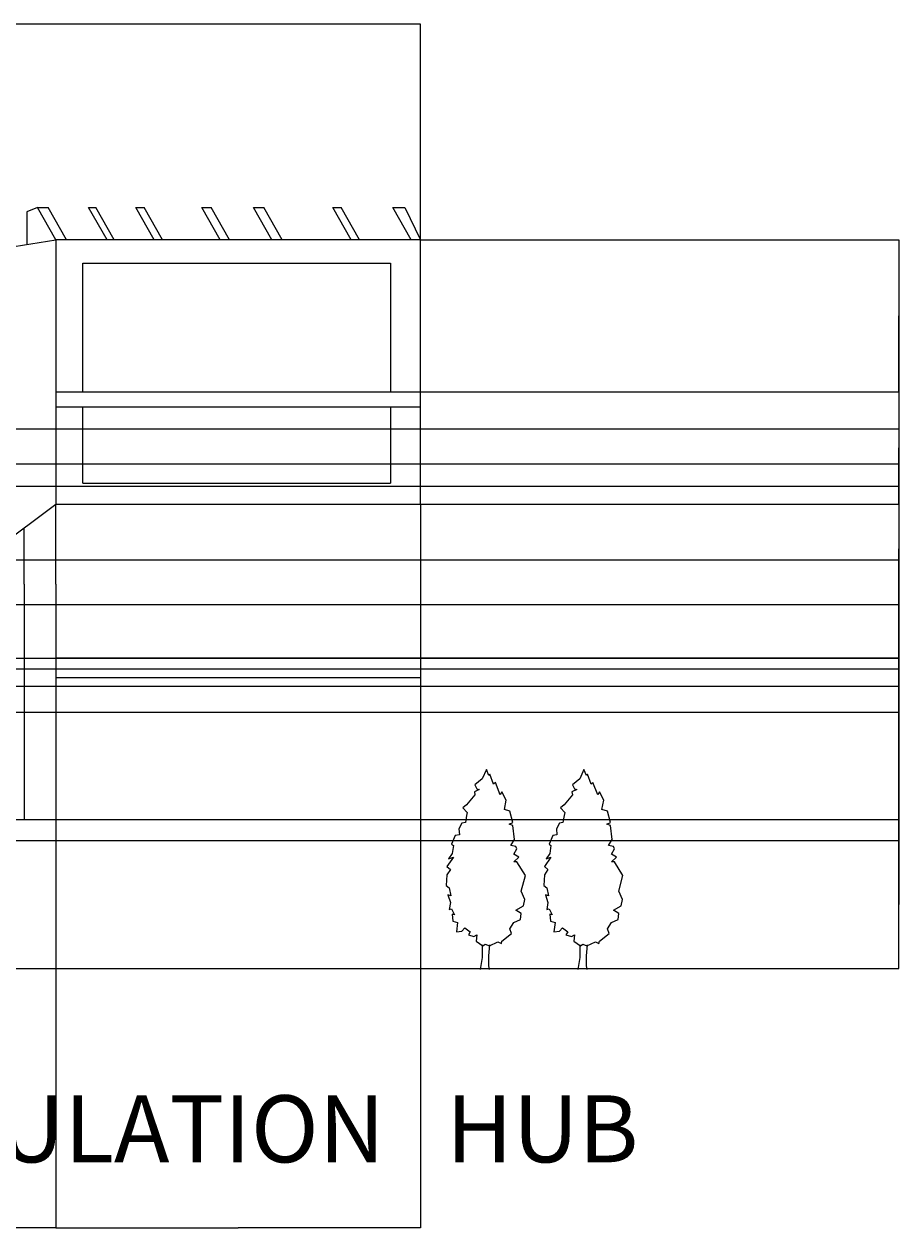
# Model space of a CAD drawing. Units: inches. Extents: x -32109 to 33221, y -19197 to 7608.
# Tile 24 of 25: x 26633 to 33221, y -13530 to -4467. Entities that reach past the tile are written whole.
import ezdxf

# ---------------------------------------------------------------- set-up
doc = ezdxf.new("R2010")
doc.units = ezdxf.units.IN
doc.header["$MEASUREMENT"] = 0
for name, color, linetype, lineweight in [('A-ANNO-DIMS', 2, 'Continuous', 18), ('A-ANNO-TEXT', 7, 'Continuous', 25), ('A-ELEV', 7, 'Continuous', 25), ('L-PLNT', 3, 'Continuous', 13)]:
    doc.layers.add(name, color=color, linetype=linetype, lineweight=lineweight)
doc.styles.get("Standard").update_dxf_attribs({"font": 'arial.ttf'})
doc.dimstyles.get("Standard").update_dxf_attribs({"dimtxt": 0.18, "dimasz": 0.18, "dimexe": 0.18, "dimexo": 0.0625, "dimgap": 0.09, "dimtad": 0, "dimtih": 1, "dimtoh": 1, "dimdec": 4, "dimzin": 0, "dimdsep": 46, "dimtxsty": 'Standard', "dimcen": 0.09, "dimadec": 0, "dimazin": 0, "dimtfac": 1, "dimtdec": 4, "dimtofl": 0, "dimtmove": 0, "dimatfit": 3, "dimfxl": 1, "dimtolj": 1, "dimtzin": 0, "dimarcsym": 0})

# ---------------------------------------------------------------- blocks, each defined once
blk = doc.blocks.new('*U2')
blk.add_lwpolyline([(-2.75400000000036, 191.699), (-6.7800000000002, 182.8509999999996), (-13.68200000000024, 176.9529999999995), (-11.95600000000013, 173.2659999999996), (-9.655999999999949, 172.529), (-14.25700000000006, 170.317), (-13.68200000000024, 167.3679999999999), (-21.73300000000017, 157.7829999999999), (-25.1840000000002, 154.8340000000003), (-21.15800000000036, 150.4099999999998), (-21.73300000000017, 147.4609999999998), (-22.88400000000001, 140.8249999999998), (-26.33400000000029, 140.087), (-29.21000000000004, 134.9259999999995), (-28.63499999999977, 129.0279999999998), (-32.66100000000006, 128.2909999999997), (-36.11099999999988, 120.1799999999998), (-34.38599999999997, 118.7059999999997), (-35.53600000000006, 111.3329999999996), (-38.98700000000008, 106.1709999999998), (-34.38599999999997, 107.6459999999997), (-40.71199999999999, 98.79799999999977), (-37.26099999999997, 95.8489999999997), (-40.71199999999999, 90.68799999999965), (-41.28700000000026, 80.36599999999999), (-38.41200000000026, 78.154), (-36.68600000000015, 70.78099999999995), (-39.5619999999999, 71.51799999999957), (-37.26099999999997, 64.14499999999998), (-38.41200000000026, 57.50899999999956), (-36.11099999999988, 58.24699999999984), (-33.23599999999988, 52.3479999999995), (-35.53600000000006, 53.08599999999978), (-34.96100000000024, 46.44999999999981), (-30.36000000000013, 44.9749999999999), (-31.50999999999977, 36.1279999999997), (-26.33400000000029, 36.86499999999978), (-23.45900000000029, 39.81399999999985), (-18.28300000000036, 36.1279999999997), (-20.00800000000027, 33.17799999999988), (-14.83199999999988, 31.70399999999972), (-11.95600000000013, 33.17799999999988), (-12.53099999999995, 27.27999999999975), (-6.204999999999927, 22.85599999999977), (-3.9050000000002, 24.33099999999968), (0.1209999999996398, 22.85599999999977), (8.172999999999774, 26.54299999999967), (11.62399999999979, 25.06799999999976), (12.19900000000007, 27.27999999999975), (21.40000000000009, 34.6529999999998), (19.67500000000018, 39.07699999999977), (23.70099999999957, 44.9749999999999), (30.02700000000004, 47.92399999999997), (30.60199999999986, 53.82299999999986), (25.42599999999993, 56.77199999999993), (32.90299999999979, 61.19599999999991), (34.05299999999988, 67.0939999999996), (30.60199999999986, 75.20499999999993), (34.6279999999997, 89.95100000000002), (26.57599999999957, 103.2219999999997), (23.70099999999957, 103.2219999999997), (28.30199999999968, 107.6459999999997), (23.70099999999957, 110.5949999999998), (26.57599999999957, 115.7559999999994), (25.42599999999993, 117.9679999999998), (20.82499999999982, 118.7059999999997), (24.27599999999984, 124.6040000000002), (22.55099999999993, 137.8759999999997), (19.09999999999991, 139.3499999999999), (22.55099999999993, 140.8249999999998), (19.67500000000018, 151.884), (14.49899999999979, 153.3589999999999), (16.22400000000016, 162.2069999999999), (12.19900000000007, 170.317), (10.47299999999995, 167.3679999999999), (5.871999999999843, 179.1649999999999), (4.146999999999934, 177.69), (0.6959999999999127, 187.2749999999996), (-0.4540000000001783, 185.7999999999997)], close=True)
for points in [[(-6.813000000000101, 23.66899999999987), (-6.813000000000101, 11.66899999999987), (-8.626999999999953, 0)], [(0.3869999999997162, 23.66899999999987), (-0.5760000000000219, 13.27099999999973), (-0.5760000000000219, 3.685999999999694), (0, 0)]]:
    blk.add_lwpolyline(points)
blk = doc.blocks.new('*D16')
at = {"layer": 'A-ANNO-DIMS', "color": 0, "lineweight": -2, "transparency": 16777216}
for p, q in [((7931.85712, -8929.002357), (7931.85712, -4467.086268999999)), ((7932.03712, -4467.266268999999), (18774.66361096794, -4467.266268999999)), ((29618.150443, -4467.266268999999), (18775.52395203206, -4467.266268999999)), ((29618.330443, -6090.731526999999), (29618.330443, -4467.086268999999))]:
    blk.add_line(p, q, dxfattribs=at)
at = {"layer": 'A-ANNO-DIMS', "color": 0, "transparency": 16777216}
for points in [[(7932.03712, -4467.236268999999), (7932.03712, -4467.296269), (7931.85712, -4467.266268999999)], [(29618.150443, -4467.236268999999), (29618.150443, -4467.296269), (29618.330443, -4467.266268999999)]]:
    blk.add_solid(points, dxfattribs=at)
at = {"layer": 'Defpoints', "color": 0, "transparency": 16777216}
for p in [(29618.330443, -4467.266268999999), (29618.330443, -6090.794027), (7931.85712, -8929.064857)]:
    blk.add_point(p, dxfattribs=at)
at = {"layer": 'A-ANNO-DIMS', "color": 0, "transparency": 16777216, "insert": (18775.0937815, -4467.266268999999), "char_height": 0.18, "attachment_point": 5}
blk.add_mtext('\\A1;21686', dxfattribs=at)
blk = doc.blocks.new('*D17')
at = {"layer": 'A-ANNO-DIMS', "color": 0, "lineweight": -2, "transparency": 16777216}
for p, q in [((29618.39294300002, -6090.794027000002), (33221.11530000003, -6090.794027000001)), ((33220.93530000003, -6090.974027000001), (33220.93530000003, -8833.116883862214)), ((33220.93530000003, -11575.623547), (33220.93530000003, -8833.48069013779)), ((8978.174905000003, -11575.803547), (33221.11530000003, -11575.803547))]:
    blk.add_line(p, q, dxfattribs=at)
at = {"layer": 'A-ANNO-DIMS', "color": 0, "transparency": 16777216}
for points in [[(33220.90530000003, -6090.974027000001), (33220.96530000003, -6090.974027000001), (33220.93530000003, -6090.794027000001)], [(33220.90530000003, -11575.623547), (33220.96530000003, -11575.623547), (33220.93530000003, -11575.803547)]]:
    blk.add_solid(points, dxfattribs=at)
at = {"layer": 'Defpoints', "color": 0, "transparency": 16777216}
for p in [(29618.33044300001, -6090.794027000002), (8978.112405000002, -11575.803547), (33220.93530000003, -11575.803547)]:
    blk.add_point(p, dxfattribs=at)
at = {"layer": 'A-ANNO-DIMS', "color": 0, "transparency": 16777216, "insert": (33220.93530000002, -8833.298787000009), "char_height": 0.18, "attachment_point": 5}
blk.add_mtext('\\A1;5485', dxfattribs=at)
blk = doc.blocks.new('*D140')
at = {"layer": 'A-ANNO-DIMS', "color": 0, "lineweight": -2, "transparency": 16777216}
for p, q in [((24779.369992, -11575.866047), (24779.369992, -13529.670166)), ((26872.591633, -11575.866047), (26872.591633, -13529.670166)), ((24779.549992, -13529.490166), (25825.51656966234, -13529.490166)), ((26872.411633, -13529.490166), (25826.44505533765, -13529.490166))]:
    blk.add_line(p, q, dxfattribs=at)
at = {"layer": 'A-ANNO-DIMS', "color": 0, "transparency": 16777216}
for points in [[(24779.549992, -13529.460166), (24779.549992, -13529.520166), (24779.369992, -13529.490166)], [(26872.411633, -13529.460166), (26872.411633, -13529.520166), (26872.591633, -13529.490166)]]:
    blk.add_solid(points, dxfattribs=at)
at = {"layer": 'Defpoints', "color": 0, "transparency": 16777216}
for p in [(24779.369992, -11575.803547), (26872.591633, -11575.803547), (26872.591633, -13529.490166)]:
    blk.add_point(p, dxfattribs=at)
at = {"layer": 'A-ANNO-DIMS', "color": 0, "transparency": 16777216, "insert": (25825.9808125, -13529.490166), "char_height": 0.18, "attachment_point": 5}
blk.add_mtext('\\A1;2093.2', dxfattribs=at)
blk = doc.blocks.new('*D141')
at = {"layer": 'A-ANNO-DIMS', "color": 0, "lineweight": -2, "transparency": 16777216}
for p, q in [((26872.591633, -11575.866047), (26872.591633, -13529.670166)), ((29618.330443, -11575.866047), (29618.330443, -13529.670166)), ((26872.771633, -13529.490166), (28245.10079243383, -13529.490166)), ((29618.150443, -13529.490166), (28245.82128356617, -13529.490166))]:
    blk.add_line(p, q, dxfattribs=at)
at = {"layer": 'A-ANNO-DIMS', "color": 0, "transparency": 16777216}
for points in [[(26872.771633, -13529.460166), (26872.771633, -13529.520166), (26872.591633, -13529.490166)], [(29618.150443, -13529.460166), (29618.150443, -13529.520166), (29618.330443, -13529.490166)]]:
    blk.add_solid(points, dxfattribs=at)
at = {"layer": 'Defpoints', "color": 0, "transparency": 16777216}
for p in [(26872.591633, -11575.803547), (29618.330443, -11575.803547), (29618.330443, -13529.490166)]:
    blk.add_point(p, dxfattribs=at)
at = {"layer": 'A-ANNO-DIMS', "color": 0, "transparency": 16777216, "insert": (28245.461038, -13529.490166), "char_height": 0.18, "attachment_point": 5}
blk.add_mtext('\\A1;2746', dxfattribs=at)
blk = doc.blocks.new('*D142')
at = {"layer": 'A-ANNO-DIMS', "color": 0, "lineweight": -2, "transparency": 16777216}
for p, q in [((19422.79326, -7777.039673000004), (33221.11530000003, -7777.039673000001)), ((33220.93530000003, -7777.219673000002), (33220.93530000003, -9676.23964547067)), ((33220.93530000003, -11575.623547), (33220.93530000003, -9676.603574529332)), ((19422.79326, -11575.803547), (33221.11530000003, -11575.803547))]:
    blk.add_line(p, q, dxfattribs=at)
at = {"layer": 'A-ANNO-DIMS', "color": 0, "transparency": 16777216}
for points in [[(33220.90530000003, -7777.219673000002), (33220.96530000003, -7777.219673000002), (33220.93530000003, -7777.039673000001)], [(33220.90530000003, -11575.623547), (33220.96530000003, -11575.623547), (33220.93530000003, -11575.803547)]]:
    blk.add_solid(points, dxfattribs=at)
at = {"layer": 'Defpoints', "color": 0, "transparency": 16777216}
for p in [(19422.73076, -7777.039673000004), (19422.73076, -11575.803547), (33220.93530000003, -11575.803547)]:
    blk.add_point(p, dxfattribs=at)
at = {"layer": 'A-ANNO-DIMS', "color": 0, "transparency": 16777216, "insert": (33220.93530000002, -9676.421610000009), "char_height": 0.18, "attachment_point": 5}
blk.add_mtext('\\A1;3799', dxfattribs=at)
blk = doc.blocks.new('*D143')
at = {"layer": 'A-ANNO-DIMS', "color": 0, "lineweight": -2, "transparency": 16777216}
for p, q in [((23344.28486700001, -9241.758819000004), (33221.11530000003, -9241.758819000002)), ((33220.93530000003, -9241.938819000003), (33220.93530000003, -10408.59921847067)), ((33220.93530000003, -11575.623547), (33220.93530000003, -10408.96314752933)), ((23344.28486700001, -11575.803547), (33221.11530000003, -11575.803547))]:
    blk.add_line(p, q, dxfattribs=at)
at = {"layer": 'A-ANNO-DIMS', "color": 0, "transparency": 16777216}
for points in [[(33220.90530000003, -9241.938819000003), (33220.96530000003, -9241.938819000003), (33220.93530000003, -9241.758819000002)], [(33220.90530000003, -11575.623547), (33220.96530000003, -11575.623547), (33220.93530000003, -11575.803547)]]:
    blk.add_solid(points, dxfattribs=at)
at = {"layer": 'Defpoints', "color": 0, "transparency": 16777216}
for p in [(23344.222367, -9241.758819000004), (23344.222367, -11575.803547), (33220.93530000003, -11575.803547)]:
    blk.add_point(p, dxfattribs=at)
at = {"layer": 'A-ANNO-DIMS', "color": 0, "transparency": 16777216, "insert": (33220.93530000002, -10408.78118300001), "char_height": 0.18, "attachment_point": 5}
blk.add_mtext('\\A1;2334', dxfattribs=at)
blk = doc.blocks.new('*D144')
at = {"layer": 'A-ANNO-DIMS', "color": 0, "lineweight": -2, "transparency": 16777216}
for p, q in [((22344.03431300001, -7946.222949000004), (33221.11530000003, -7946.222949000001)), ((33220.93530000003, -7946.402949000002), (33220.93530000003, -8593.808980862214)), ((33220.93530000003, -9241.578819000002), (33220.93530000003, -8594.172787137792)), ((22344.03431300001, -9241.758819000004), (33221.11530000003, -9241.758819000002))]:
    blk.add_line(p, q, dxfattribs=at)
at = {"layer": 'A-ANNO-DIMS', "color": 0, "transparency": 16777216}
for points in [[(33220.90530000003, -7946.402949000002), (33220.96530000003, -7946.402949000002), (33220.93530000003, -7946.222949000001)], [(33220.90530000003, -9241.578819000002), (33220.96530000003, -9241.578819000002), (33220.93530000003, -9241.758819000002)]]:
    blk.add_solid(points, dxfattribs=at)
at = {"layer": 'Defpoints', "color": 0, "transparency": 16777216}
for p in [(22343.97181300001, -7946.222949000004), (22343.97181300001, -9241.758819000004), (33220.93530000003, -9241.758819000002)]:
    blk.add_point(p, dxfattribs=at)
at = {"layer": 'A-ANNO-DIMS', "color": 0, "transparency": 16777216, "insert": (33220.93530000002, -8593.99088400001), "char_height": 0.18, "attachment_point": 5}
blk.add_mtext('\\A1;1295.5', dxfattribs=at)
blk = doc.blocks.new('*D145')
at = {"layer": 'A-ANNO-DIMS', "color": 0, "lineweight": -2, "transparency": 16777216}
for p, q in [((20542.28536700001, -9450.896666000002), (33221.11530000003, -9450.896666000002)), ((33220.93530000003, -9451.076666000004), (33220.93530000003, -10513.16820336221)), ((33220.93530000003, -11575.623547), (33220.93530000003, -10513.53200963779)), ((20542.28536700001, -11575.803547), (33221.11530000003, -11575.803547))]:
    blk.add_line(p, q, dxfattribs=at)
at = {"layer": 'A-ANNO-DIMS', "color": 0, "transparency": 16777216}
for points in [[(33220.90530000003, -9451.076666000004), (33220.96530000003, -9451.076666000004), (33220.93530000003, -9450.896666000002)], [(33220.90530000003, -11575.623547), (33220.96530000003, -11575.623547), (33220.93530000003, -11575.803547)]]:
    blk.add_solid(points, dxfattribs=at)
at = {"layer": 'Defpoints', "color": 0, "transparency": 16777216}
for p in [(20542.22286700001, -9450.896666000002), (20542.22286700001, -11575.803547), (33220.93530000003, -11575.803547)]:
    blk.add_point(p, dxfattribs=at)
at = {"layer": 'A-ANNO-DIMS', "color": 0, "transparency": 16777216, "insert": (33220.93530000002, -10513.35010650001), "char_height": 0.18, "attachment_point": 5}
blk.add_mtext('\\A1;2125', dxfattribs=at)
blk = doc.blocks.new('*D147')
at = {"layer": 'A-ANNO-DIMS', "color": 0, "lineweight": -2, "transparency": 16777216}
for p, q in [((25729.07058000001, -7514.357851000004), (33221.11530000003, -7514.357851000003)), ((33220.93530000003, -7514.537851000003), (33220.93530000003, -8416.924501362213)), ((33220.93530000003, -9319.674958000001), (33220.93530000003, -8417.288307637791)), ((23373.8343, -9319.854958000004), (33221.11530000003, -9319.854958000002))]:
    blk.add_line(p, q, dxfattribs=at)
at = {"layer": 'A-ANNO-DIMS', "color": 0, "transparency": 16777216}
for points in [[(33220.90530000003, -7514.537851000003), (33220.96530000003, -7514.537851000003), (33220.93530000003, -7514.357851000003)], [(33220.90530000003, -9319.674958000001), (33220.96530000003, -9319.674958000001), (33220.93530000003, -9319.854958000002)]]:
    blk.add_solid(points, dxfattribs=at)
at = {"layer": 'Defpoints', "color": 0, "transparency": 16777216}
for p in [(25729.00808000002, -7514.357851000004), (33220.93530000003, -7514.357851000003), (23373.77180000001, -9319.854958000004)]:
    blk.add_point(p, dxfattribs=at)
at = {"layer": 'A-ANNO-DIMS', "color": 0, "transparency": 16777216, "insert": (33220.93530000002, -8417.10640450001), "char_height": 0.18, "attachment_point": 5}
blk.add_mtext('\\A1;1805.5', dxfattribs=at)
blk = doc.blocks.new('*D149')
at = {"layer": 'A-ANNO-DIMS', "color": 0, "lineweight": -2, "transparency": 16777216}
for p, q in [((24743.24553300002, -8499.326661000003), (33221.11530000003, -8499.326661000001)), ((33220.93530000003, -8499.506661000001), (33220.93530000003, -8667.240442470671)), ((33220.93530000003, -8835.338153000002), (33220.93530000003, -8667.604371529334)), ((24743.24553300002, -8835.518153000005), (33221.11530000003, -8835.518153000003))]:
    blk.add_line(p, q, dxfattribs=at)
at = {"layer": 'A-ANNO-DIMS', "color": 0, "transparency": 16777216}
for points in [[(33220.90530000003, -8499.506661000001), (33220.96530000003, -8499.506661000001), (33220.93530000003, -8499.326661000001)], [(33220.90530000003, -8835.338153000002), (33220.96530000003, -8835.338153000002), (33220.93530000003, -8835.518153000003)]]:
    blk.add_solid(points, dxfattribs=at)
at = {"layer": 'Defpoints', "color": 0, "transparency": 16777216}
for p in [(24743.18303300002, -8499.326661000003), (33220.93530000003, -8499.326661000001), (24743.18303300002, -8835.518153000005)]:
    blk.add_point(p, dxfattribs=at)
at = {"layer": 'A-ANNO-DIMS', "color": 0, "transparency": 16777216, "insert": (33220.93530000002, -8667.422407000007), "char_height": 0.18, "attachment_point": 5}
blk.add_mtext('\\A1;336.2', dxfattribs=at)
blk = doc.blocks.new('*D150')
at = {"layer": 'A-ANNO-DIMS', "color": 0, "lineweight": -2, "transparency": 16777216}
for p, q in [((24779.43249200002, -9646.283758000003), (33221.11530000003, -9646.283758000001)), ((33220.93530000003, -9646.463758000002), (33220.93530000003, -10050.72724947067)), ((33220.93530000003, -10455.35467), (33220.93530000003, -10051.09117852933)), ((24779.43249200002, -10455.53467), (33221.11530000003, -10455.53467))]:
    blk.add_line(p, q, dxfattribs=at)
at = {"layer": 'A-ANNO-DIMS', "color": 0, "transparency": 16777216}
for points in [[(33220.90530000003, -9646.463758000002), (33220.96530000003, -9646.463758000002), (33220.93530000003, -9646.283758000001)], [(33220.90530000003, -10455.35467), (33220.96530000003, -10455.35467), (33220.93530000003, -10455.53467)]]:
    blk.add_solid(points, dxfattribs=at)
at = {"layer": 'Defpoints', "color": 0, "transparency": 16777216}
for p in [(24779.36999200001, -9646.283758000003), (24779.36999200001, -10455.53467), (33220.93530000003, -10455.53467)]:
    blk.add_point(p, dxfattribs=at)
at = {"layer": 'A-ANNO-DIMS', "color": 0, "transparency": 16777216, "insert": (33220.93530000002, -10050.90921400001), "char_height": 0.18, "attachment_point": 5}
blk.add_mtext('\\A1;809.3', dxfattribs=at)
blk = doc.blocks.new('*D151')
at = {"layer": 'A-ANNO-DIMS', "color": 0, "lineweight": -2, "transparency": 16777216}
for p, q in [((24779.43249200002, -10455.53467), (33221.11530000003, -10455.53467)), ((33220.93530000003, -10455.71467), (33220.93530000003, -11015.48714397067)), ((33220.93530000003, -11575.623547), (33220.93530000003, -11015.85107302933)), ((24779.43249200002, -11575.803547), (33221.11530000003, -11575.803547))]:
    blk.add_line(p, q, dxfattribs=at)
at = {"layer": 'A-ANNO-DIMS', "color": 0, "transparency": 16777216}
for points in [[(33220.90530000003, -10455.71467), (33220.96530000003, -10455.71467), (33220.93530000003, -10455.53467)], [(33220.90530000003, -11575.623547), (33220.96530000003, -11575.623547), (33220.93530000003, -11575.803547)]]:
    blk.add_solid(points, dxfattribs=at)
at = {"layer": 'Defpoints', "color": 0, "transparency": 16777216}
for p in [(24779.36999200001, -10455.53467), (24779.36999200001, -11575.803547), (33220.93530000003, -11575.803547)]:
    blk.add_point(p, dxfattribs=at)
at = {"layer": 'A-ANNO-DIMS', "color": 0, "transparency": 16777216, "insert": (33220.93530000002, -11015.66910850001), "char_height": 0.18, "attachment_point": 5}
blk.add_mtext('\\A1;1120.3', dxfattribs=at)
blk = doc.blocks.new('*D153')
at = {"layer": 'A-ANNO-DIMS', "color": 0, "lineweight": -2, "transparency": 16777216}
for p, q in [((29618.39294300002, -10614.330461), (33221.11530000003, -10614.330461)), ((33220.93530000003, -10614.510461), (33220.93530000003, -11094.88510086221)), ((33220.93530000003, -11575.623547), (33220.93530000003, -11095.24890713779)), ((29618.39294300002, -11575.803547), (33221.11530000003, -11575.803547))]:
    blk.add_line(p, q, dxfattribs=at)
at = {"layer": 'A-ANNO-DIMS', "color": 0, "transparency": 16777216}
for points in [[(33220.90530000003, -10614.510461), (33220.96530000003, -10614.510461), (33220.93530000003, -10614.330461)], [(33220.90530000003, -11575.623547), (33220.96530000003, -11575.623547), (33220.93530000003, -11575.803547)]]:
    blk.add_solid(points, dxfattribs=at)
at = {"layer": 'Defpoints', "color": 0, "transparency": 16777216}
for p in [(29618.33044300001, -10614.330461), (33220.93530000003, -10614.330461), (29618.33044300001, -11575.803547)]:
    blk.add_point(p, dxfattribs=at)
at = {"layer": 'A-ANNO-DIMS', "color": 0, "transparency": 16777216, "insert": (33220.93530000002, -11095.06700400001), "char_height": 0.18, "attachment_point": 5}
blk.add_mtext('\\A1;961.5', dxfattribs=at)
blk = doc.blocks.new('*D154')
at = {"layer": 'A-ANNO-DIMS', "color": 0, "lineweight": -2, "transparency": 16777216}
for p, q in [((29618.39294300002, -9238.017771000004), (33221.11530000003, -9238.017771000004)), ((33220.93530000003, -9238.197771000005), (33220.93530000003, -9925.992151470673)), ((33220.93530000003, -10614.150461), (33220.93530000003, -9926.356080529336)), ((29618.39294300002, -10614.330461), (33221.11530000003, -10614.330461))]:
    blk.add_line(p, q, dxfattribs=at)
at = {"layer": 'A-ANNO-DIMS', "color": 0, "transparency": 16777216}
for points in [[(33220.90530000003, -9238.197771000005), (33220.96530000003, -9238.197771000005), (33220.93530000003, -9238.017771000004)], [(33220.90530000003, -10614.150461), (33220.96530000003, -10614.150461), (33220.93530000003, -10614.330461)]]:
    blk.add_solid(points, dxfattribs=at)
at = {"layer": 'Defpoints', "color": 0, "transparency": 16777216}
for p in [(29618.33044300001, -9238.017771000004), (33220.93530000003, -9238.017771000004), (29618.33044300001, -10614.330461)]:
    blk.add_point(p, dxfattribs=at)
at = {"layer": 'A-ANNO-DIMS', "color": 0, "transparency": 16777216, "insert": (33220.93530000002, -9926.174116000013), "char_height": 0.18, "attachment_point": 5}
blk.add_mtext('\\A1;1376.3', dxfattribs=at)
blk = doc.blocks.new('*D155')
at = {"layer": 'A-ANNO-DIMS', "color": 0, "lineweight": -2, "transparency": 16777216}
for p, q in [((29618.39294300002, -8080.142133000004), (33221.11530000003, -8080.142133000002)), ((33220.93530000003, -8080.322133000002), (33220.93530000003, -8658.898048862215)), ((33220.93530000003, -9237.837771000004), (33220.93530000003, -8659.261855137793)), ((29618.39294300002, -9238.017771000004), (33221.11530000003, -9238.017771000004))]:
    blk.add_line(p, q, dxfattribs=at)
at = {"layer": 'A-ANNO-DIMS', "color": 0, "transparency": 16777216}
for points in [[(33220.90530000003, -8080.322133000002), (33220.96530000003, -8080.322133000002), (33220.93530000003, -8080.142133000002)], [(33220.90530000003, -9237.837771000004), (33220.96530000003, -9237.837771000004), (33220.93530000003, -9238.017771000004)]]:
    blk.add_solid(points, dxfattribs=at)
at = {"layer": 'Defpoints', "color": 0, "transparency": 16777216}
for p in [(29618.33044300001, -8080.142133000004), (33220.93530000003, -8080.142133000002), (29618.33044300001, -9238.017771000004)]:
    blk.add_point(p, dxfattribs=at)
at = {"layer": 'A-ANNO-DIMS', "color": 0, "transparency": 16777216, "insert": (33220.93530000002, -8659.079952000011), "char_height": 0.18, "attachment_point": 5}
blk.add_mtext('\\A1;1157.9', dxfattribs=at)
blk = doc.blocks.new('*D156')
at = {"layer": 'A-ANNO-DIMS', "color": 0, "lineweight": -2, "transparency": 16777216}
for p, q in [((29618.39294300002, -7235.783167000004), (33221.11530000003, -7235.783167000002)), ((33220.93530000003, -7235.963167000003), (33220.93530000003, -7657.780746862214)), ((33220.93530000003, -8079.962133000002), (33220.93530000003, -7658.144553137794)), ((29618.39294300002, -8080.142133000004), (33221.11530000003, -8080.142133000002))]:
    blk.add_line(p, q, dxfattribs=at)
at = {"layer": 'A-ANNO-DIMS', "color": 0, "transparency": 16777216}
for points in [[(33220.90530000003, -7235.963167000003), (33220.96530000003, -7235.963167000003), (33220.93530000003, -7235.783167000002)], [(33220.90530000003, -8079.962133000002), (33220.96530000003, -8079.962133000002), (33220.93530000003, -8080.142133000002)]]:
    blk.add_solid(points, dxfattribs=at)
at = {"layer": 'Defpoints', "color": 0, "transparency": 16777216}
for p in [(29618.33044300001, -7235.783167000004), (33220.93530000003, -7235.783167000002), (29618.33044300001, -8080.142133000004)]:
    blk.add_point(p, dxfattribs=at)
at = {"layer": 'A-ANNO-DIMS', "color": 0, "transparency": 16777216, "insert": (33220.93530000002, -7657.96265000001), "char_height": 0.18, "attachment_point": 5}
blk.add_mtext('\\A1;844.4', dxfattribs=at)
blk = doc.blocks.new('*D157')
at = {"layer": 'A-ANNO-DIMS', "color": 0, "lineweight": -2, "transparency": 16777216}
for p, q in [((29618.39294300002, -6090.794027000002), (33221.11530000003, -6090.794027000001)), ((33220.93530000003, -6090.974027000001), (33220.93530000003, -6663.106693862212)), ((33220.93530000003, -7235.603167000002), (33220.93530000003, -6663.470500137792)), ((29618.39294300002, -7235.783167000004), (33221.11530000003, -7235.783167000002))]:
    blk.add_line(p, q, dxfattribs=at)
at = {"layer": 'A-ANNO-DIMS', "color": 0, "transparency": 16777216}
for points in [[(33220.90530000003, -6090.974027000001), (33220.96530000003, -6090.974027000001), (33220.93530000003, -6090.794027000001)], [(33220.90530000003, -7235.603167000002), (33220.96530000003, -7235.603167000002), (33220.93530000003, -7235.783167000002)]]:
    blk.add_solid(points, dxfattribs=at)
at = {"layer": 'Defpoints', "color": 0, "transparency": 16777216}
for p in [(29618.33044300001, -6090.794027000002), (33220.93530000003, -6090.794027000001), (29618.33044300001, -7235.783167000004)]:
    blk.add_point(p, dxfattribs=at)
at = {"layer": 'A-ANNO-DIMS', "color": 0, "transparency": 16777216, "insert": (33220.93530000002, -6663.28859700001), "char_height": 0.18, "attachment_point": 5}
blk.add_mtext('\\A1;1145', dxfattribs=at)

msp = doc.modelspace()

# ---------------------------------------------------------------- linework, layer by layer
at = {"layer": 'A-ELEV'}
for p, q in [((26734.30131227388, -5847.266268706711), (26653.99030379239, -5881.151844908814)), ((26653.99030379239, -5881.151844908814), (26653.99030379239, -6125.338823921676)), ((26872.5916333869, -6090.794027193029), (26734.30131227388, -5847.266268706711)), ((26734.30131227388, -5847.266268706711), (26814.41404308503, -5847.266268706711)), ((26952.70436419804, -6090.794027193029), (26814.41404308503, -5847.266268706711)), ((27118.91956764719, -5847.266268706711), (27173.22604034306, -5847.266268706711)), ((27257.2098887602, -6090.794027193029), (27118.91956764719, -5847.266268706711)), ((27311.51636145608, -6090.794027193029), (27173.22604034306, -5847.266268706711)), ((27474.65123435393, -5847.266268706711), (27536.29579281685, -5847.266268706711)), ((27612.94155546695, -6090.794027193029), (27474.65123435393, -5847.266268706711)), ((27674.58611392986, -6090.794027193029), (27536.29579281685, -5847.266268706711)), ((27972.30789923587, -5847.266268706711), (28042.13039404891, -5847.266268706711)), ((28110.59822034889, -6090.794027193029), (27972.30789923587, -5847.266268706711)), ((28180.42071516193, -6090.794027193029), (28042.13039404891, -5847.266268706711)), ((28360.79031287655, -5847.266268706711), (28437.84574743128, -5847.266268706711)), ((28499.08063398956, -6090.794027193029), (28360.79031287655, -5847.266268706711)), ((28576.1360685443, -6090.794027193029), (28437.84574743128, -5847.266268706711)), ((28957.58334115401, -5847.266268706711), (29019.64795667042, -5847.266268706711)), ((29095.87366226702, -6090.794027193029), (28957.583341154, -5847.266268706711)), ((29157.93827778344, -6090.794027193029), (29019.64795667042, -5847.266268706711)), ((29408.74596207834, -5847.266268706711), (29499.47233230953, -5847.266268706711)), ((29547.03628319136, -6090.794027193029), (29408.74596207834, -5847.266268706711)), ((29499.47233230953, -5847.266268706711), (29618.33044309968, -6090.794027193029)), ((25757.25718631681, -6267.046394138653), (26872.59163338689, -6090.794027193029)), ((26872.59163338689, -6090.794027193029), (26872.59163338689, -8080.14213313484)), ((29618.33044309967, -6090.794027193029), (26872.59163338689, -6090.794027193029)), ((29618.33044309968, -8080.14213313484), (29618.33044309967, -6090.794027193029)), ((27076.07005626783, -6265.751348465259), (29392.902864227, -6265.751348465259)), ((27076.07005626783, -7235.783167175667), (27076.07005626783, -6265.751348465259)), ((27532.36069853955, -6265.751348465262), (27957.14247158767, -6265.751348465262)), ((29392.902864227, -6265.751348465259), (29392.902864227, -7235.783167175667)), ((26872.5916333869, -7235.783167175667), (29618.33044309968, -7235.783167175667)), ((26872.5916333869, -7348.289835785934), (29618.33044309968, -7348.289835785934)), ((27076.07005626783, -7924.125437767102), (27076.07005626783, -7348.289835785934)), ((29392.902864227, -7348.289835785934), (29392.902864227, -7924.125437767102)), ((27076.07005626783, -7924.125437767102), (29392.902864227, -7924.125437767102)), ((24779.36999243395, -9646.283757557641), (26872.5916333869, -8080.142133134835)), ((26872.59163338689, -8080.14213313484), (27076.07005626783, -8080.14213313484)), ((26872.59163338689, -8080.14213313484), (29618.33044309968, -8080.14213313484)), ((26872.59163338689, -8684.172668917163), (26872.59163338689, -8080.14213313484)), ((29392.902864227, -8080.14213313484), (29618.33044309968, -8080.14213313484)), ((29618.33044309968, -8080.142133134835), (29618.33044309985, -11575.80354668385)), ((26632.5501278899, -8684.172668917163), (26632.5501278899, -8259.740406911897)), ((26632.5501278899, -8684.172668917163), (26632.5501278899, -9646.283757557647)), ((26872.59163338689, -8684.172668917163), (26872.59163338688, -9646.283757557647)), ((26872.59163338688, -9238.017770679995), (29618.33044309975, -9238.017770679991)), ((26872.59163338688, -9384.951678068028), (29618.33044309975, -9384.951678068024)), ((26632.55012788991, -9646.283757557641), (26632.5501278899, -10455.53467010263)), ((26872.5916333869, -9646.283757557641), (26872.59163338689, -11575.80354668384)), ((26872.59163338689, -10455.53467010263), (29618.3304430998, -10455.53467010263)), ((24779.36999243395, -10614.3304611299), (27330.3209813765, -10614.3304611299)), ((26872.59163338688, -10614.3304611299), (29618.33044309975, -10614.3304611299)), ((6605.539725432871, -11575.80354668384), (31840.93529984972, -11575.80354668384)), ((20871.06445360743, -11575.80354668384), (28549.41971044784, -11575.80354668384)), ((28549.41971044784, -11575.80354668384), (29618.33044309985, -11575.80354668385))]:
    msp.add_line(p, q, dxfattribs=at)

# ---------------------------------------------------------------- block references
at = {"layer": 'L-PLNT', "xscale": 7.857670648127824, "yscale": 7.857670648127824, "zscale": 7.857670648127824}
for p in [(30135.93713987054, -11584.62579577021), (30870.68112838949, -11584.62579577021)]:
    msp.add_blockref('*U2', p, dxfattribs=at)

# ---------------------------------------------------------------- texts
at = {"layer": 'A-ANNO-TEXT'}
msp.add_text('SIDE  PROFILE   ATRIUM   CIRCULATION   AND   VERTICAL   CIRCULATION   HUB', height=504.218310670369, dxfattribs=at).set_placement((6653.0921668488, -13035.81166412015))

# ---------------------------------------------------------------- dimensions: what is measured, and where the dimension line sits
at = {"layer": 'A-ANNO-DIMS'}
for base, p1, p2, override, picture, middle in [((29618.330443, -4467.266268999999), (7931.85712, -8929.064857), (29618.330443, -6090.794027), {"dimdec": 0, "dimlfac": 1, "dimrnd": 0, "dimzin": 0, "dimdsep": 46, "dimlunit": 2}, '*D16', (18775.0937815, -4467.266268999999)), ((26872.591633, -13529.490166), (24779.369992, -11575.803547), (26872.591633, -11575.803547), {"dimdec": 1, "dimlfac": 1, "dimrnd": 0, "dimzin": 0, "dimdsep": 46, "dimlunit": 2}, '*D140', (25825.9808125, -13529.490166)), ((29618.330443, -13529.490166), (26872.591633, -11575.803547), (29618.330443, -11575.803547), {"dimdec": 0, "dimlfac": 1, "dimrnd": 0, "dimzin": 0, "dimdsep": 46, "dimlunit": 2}, '*D141', (28245.461038, -13529.490166))]:
    dim = msp.add_linear_dim(base=base, p1=p1, p2=p2, dimstyle='Standard', override=override, dxfattribs=at)
    dim.commit()
    dim.dimension.update_dxf_attribs({"geometry": picture, "text_midpoint": middle})
for base, p1, p2, override, picture, middle in [((33220.93530000003, -11575.803547), (29618.330443, -6090.794027), (8978.112405, -11575.803547), {"dimdec": 0, "dimlfac": 1, "dimrnd": 0, "dimzin": 0, "dimdsep": 46, "dimlunit": 2}, '*D17', (33220.93530000002, -8833.298787000009)), ((33220.93530000003, -6090.794027000001), (29618.330443, -7235.783167), (29618.330443, -6090.794027), {"dimdec": 0, "dimlfac": 1, "dimrnd": 0, "dimzin": 0, "dimdsep": 46, "dimlunit": 2}, '*D157', (33220.93530000002, -6663.28859700001)), ((33220.93530000003, -7235.783167000002), (29618.330443, -8080.142133), (29618.330443, -7235.783167), {"dimdec": 1, "dimlfac": 1, "dimrnd": 0, "dimzin": 0, "dimdsep": 46, "dimlunit": 2}, '*D156', (33220.93530000002, -7657.96265000001)), ((33220.93530000003, -7514.357851000003), (23373.7718, -9319.854958), (25729.00808, -7514.357850999999), {"dimdec": 1, "dimlfac": 1, "dimrnd": 0, "dimzin": 0, "dimdsep": 46, "dimlunit": 2}, '*D147', (33220.93530000002, -8417.10640450001)), ((33220.93530000003, -11575.803547), (19422.73076, -7777.039673), (19422.73076, -11575.803547), {"dimdec": 0, "dimlfac": 1, "dimrnd": 0, "dimzin": 0, "dimdsep": 46, "dimlunit": 2}, '*D142', (33220.93530000002, -9676.421610000009)), ((33220.93530000003, -9241.758819000002), (22343.971813, -7946.222949), (22343.971813, -9241.758819), {"dimdec": 1, "dimlfac": 1, "dimrnd": 0, "dimzin": 0, "dimdsep": 46, "dimlunit": 2}, '*D144', (33220.93530000002, -8593.99088400001)), ((33220.93530000003, -8080.142133000002), (29618.330443, -9238.017771), (29618.330443, -8080.142133), {"dimdec": 1, "dimlfac": 1, "dimrnd": 0, "dimzin": 0, "dimdsep": 46, "dimlunit": 2}, '*D155', (33220.93530000002, -8659.079952000011)), ((33220.93530000003, -8499.326661000001), (24743.183033, -8835.518153), (24743.183033, -8499.326661), {"dimdec": 1, "dimlfac": 1, "dimrnd": 0, "dimzin": 0, "dimdsep": 46, "dimlunit": 2}, '*D149', (33220.93530000002, -8667.422407000007)), ((33220.93530000003, -11575.803547), (23344.222367, -9241.758819), (23344.222367, -11575.803547), {"dimdec": 0, "dimlfac": 1, "dimrnd": 0, "dimzin": 0, "dimdsep": 46, "dimlunit": 2}, '*D143', (33220.93530000002, -10408.78118300001)), ((33220.93530000003, -9238.017771000004), (29618.330443, -10614.330461), (29618.330443, -9238.017771), {"dimdec": 1, "dimlfac": 1, "dimrnd": 0, "dimzin": 0, "dimdsep": 46, "dimlunit": 2}, '*D154', (33220.93530000002, -9926.174116000013)), ((33220.93530000003, -11575.803547), (20542.222867, -9450.896666), (20542.222867, -11575.803547), {"dimdec": 0, "dimlfac": 1, "dimrnd": 0, "dimzin": 0, "dimdsep": 46, "dimlunit": 2}, '*D145', (33220.93530000002, -10513.35010650001)), ((33220.93530000003, -10455.53467), (24779.369992, -9646.283758), (24779.369992, -10455.53467), {"dimdec": 1, "dimlfac": 1, "dimrnd": 0, "dimzin": 0, "dimdsep": 46, "dimlunit": 2}, '*D150', (33220.93530000002, -10050.90921400001)), ((33220.93530000003, -11575.803547), (24779.369992, -10455.53467), (24779.369992, -11575.803547), {"dimdec": 1, "dimlfac": 1, "dimrnd": 0, "dimzin": 0, "dimdsep": 46, "dimlunit": 2}, '*D151', (33220.93530000002, -11015.66910850001)), ((33220.93530000003, -10614.330461), (29618.330443, -11575.803547), (29618.330443, -10614.330461), {"dimdec": 1, "dimlfac": 1, "dimrnd": 0, "dimzin": 0, "dimdsep": 46, "dimlunit": 2}, '*D153', (33220.93530000002, -11095.06700400001))]:
    dim = msp.add_linear_dim(base=base, p1=p1, p2=p2, angle=90, dimstyle='Standard', override=override, dxfattribs=at)
    dim.commit()
    dim.dimension.update_dxf_attribs({"geometry": picture, "text_midpoint": middle})

doc.saveas('drawing.dxf')
